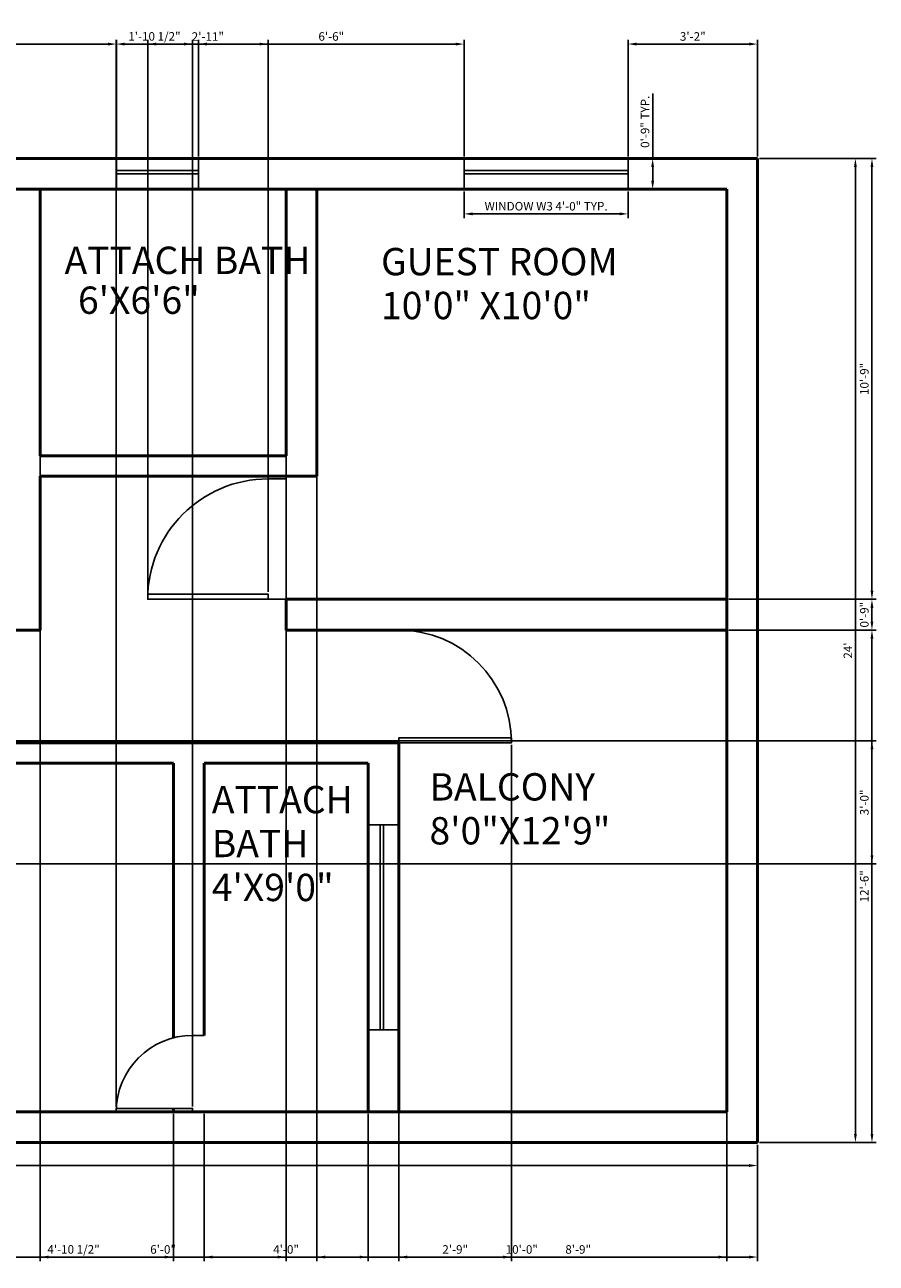
# Model space of a CAD drawing. Units: inches. Extents: x -5798 to 2718, y 1530 to 38999.
# Tile 2 of 4: x 2468 to 2718, y 1557 to 1919. Entities that reach past the tile are written whole.
import ezdxf

# ---------------------------------------------------------------- set-up
doc = ezdxf.new("R2010")
doc.units = ezdxf.units.IN
for name, color, linetype, lineweight in [('A-ANNO-DIMS', 2, 'Continuous', 18), ('A-AREA-IDEN', 3, 'Continuous', 18), ('A-DOOR', 3, 'Continuous', 25), ('A-GLAZ', 4, 'Continuous', 25), ('A-WALL', 7, 'Continuous', 50)]:
    doc.layers.add(name, color=color, linetype=linetype, lineweight=lineweight)
doc.styles.get("Standard").update_dxf_attribs({"font": 'arial.ttf'})
doc.dimstyles.new('Copy of ISO-25', dxfattribs={"dimtxt": 2.5, "dimasz": 2.5, "dimexe": 1.25, "dimexo": 0.625, "dimtad": 1, "dimdec": 1, "dimlunit": 4, "dimtxsty": 'Standard', "dimcen": 2.5, "dimadec": 0, "dimazin": 0, "dimtfac": 1, "dimtdec": 1, "dimtmove": 0, "dimatfit": 3, "dimfxl": 1, "dimarcsym": 0})

# ---------------------------------------------------------------- blocks, each defined once
blk = doc.blocks.new('*U2')
for p, q in [((0, 0), (0, -6)), ((40, 0), (40, -6))]:
    blk.add_line(p, q)
blk.add_lwpolyline([(0, 0), (0, 40), (1.75, 40), (1.75, 0)], close=True)
blk.add_arc((0, 0), 40, 0, 90)
blk = doc.blocks.new('*U7')
for p, q in [((0, 0), (0, 6)), ((40, 0), (40, 6))]:
    blk.add_line(p, q)
blk.add_lwpolyline([(0, 0), (0, -40), (1.75, -40), (1.75, 0)], close=True)
blk.add_arc((0, 0), 40, 270, 0)
blk = doc.blocks.new('*D15')
at = {"layer": 'A-ANNO-DIMS', "color": 0, "lineweight": -2, "transparency": 16777216}
for p, q in [((2683.52, 1880.03), (2712.8, 1880.03)), ((2711.55, 1877.53), (2711.55, 1594.53)), ((2683.52, 1592.03), (2712.8, 1592.03))]:
    blk.add_line(p, q, dxfattribs=at)
at = {"layer": 'A-ANNO-DIMS', "color": 0, "transparency": 16777216}
for points in [[(2711.14, 1877.53), (2711.97, 1877.53), (2711.55, 1880.03)], [(2711.14, 1594.53), (2711.97, 1594.53), (2711.55, 1592.03)]]:
    blk.add_solid(points, dxfattribs=at)
at = {"layer": 'Defpoints', "color": 0, "transparency": 16777216}
for p in [(2682.89, 1880.03), (2682.89, 1592.03), (2711.55, 1592.03)]:
    blk.add_point(p, dxfattribs=at)
at = {"layer": 'A-ANNO-DIMS', "color": 0, "transparency": 16777216, "insert": (2709.67, 1736.03), "char_height": 2.5, "attachment_point": 5, "rotation": 90}
blk.add_mtext("24'", dxfattribs=at)
blk = doc.blocks.new('*D16')
at = {"layer": 'A-ANNO-DIMS', "color": 0, "lineweight": -2, "transparency": 16777216}
for p, q in [((2042.98, 1591.41), (2042.98, 1584.06)), ((2682.89, 1591.41), (2682.89, 1584.06)), ((2045.48, 1585.31), (2680.39, 1585.31))]:
    blk.add_line(p, q, dxfattribs=at)
at = {"layer": 'A-ANNO-DIMS', "color": 0, "transparency": 16777216}
for points in [[(2045.48, 1585.73), (2045.48, 1584.89), (2042.98, 1585.31)], [(2680.39, 1585.73), (2680.39, 1584.89), (2682.89, 1585.31)]]:
    blk.add_solid(points, dxfattribs=at)
at = {"layer": 'Defpoints', "color": 0, "transparency": 16777216}
for p in [(2042.98, 1592.03), (2682.89, 1592.03), (2682.89, 1585.31)]:
    blk.add_point(p, dxfattribs=at)
at = {"layer": 'A-ANNO-DIMS', "color": 0, "transparency": 16777216, "insert": (2362.93, 1587.21), "char_height": 2.5, "attachment_point": 5}
blk.add_mtext('53\'-4"', dxfattribs=at)
blk = doc.blocks.new('WIN-48')
for p, q in [((0, 0), (0, 9)), ((0, 9), (48, 9)), ((48, 9), (48, 0)), ((0, 5.5), (48, 5.5)), ((0, 4.5), (48, 4.5))]:
    blk.add_line(p, q)
blk = doc.blocks.new('WIN-60')
for p, q in [((0, 0), (0, 9)), ((0, 9), (60, 9)), ((60, 9), (60, 0)), ((0, 4.5), (60, 4.5)), ((0, 3.5), (60, 3.5))]:
    blk.add_line(p, q)
blk = doc.blocks.new('WIN-24-B')
for p, q in [((0, 0), (0, 9)), ((0, 9), (24, 9)), ((24, 9), (24, 0)), ((0, 5.5), (24, 5.5)), ((0, 4.5), (24, 4.5))]:
    blk.add_line(p, q)
blk = doc.blocks.new('*D26')
at = {"layer": 'A-ANNO-DIMS', "color": 0, "lineweight": -2, "transparency": 16777216}
for p, q in [((2597, 1870.41), (2597, 1862.58)), ((2645, 1870.41), (2645, 1862.58)), ((2599.5, 1863.83), (2642.5, 1863.83))]:
    blk.add_line(p, q, dxfattribs=at)
at = {"layer": 'A-ANNO-DIMS', "color": 0, "transparency": 16777216}
for points in [[(2599.5, 1864.25), (2599.5, 1863.41), (2597, 1863.83)], [(2642.5, 1864.25), (2642.5, 1863.41), (2645, 1863.83)]]:
    blk.add_solid(points, dxfattribs=at)
at = {"layer": 'Defpoints', "color": 0, "transparency": 16777216}
for p in [(2597, 1871.03), (2645, 1871.03), (2645, 1863.83)]:
    blk.add_point(p, dxfattribs=at)
at = {"layer": 'A-ANNO-DIMS', "color": 0, "transparency": 16777216, "insert": (2621, 1865.75), "char_height": 2.5, "attachment_point": 5}
blk.add_mtext('WINDOW W3 4\'-0" TYP.', dxfattribs=at)
blk = doc.blocks.new('*D27')
at = {"layer": 'A-ANNO-DIMS', "color": 0, "lineweight": -2, "transparency": 16777216}
for p, q in [((2652.2, 1880.03), (2652.2, 1899.02)), ((2645.62, 1880.03), (2653.45, 1880.03)), ((2652.2, 1873.53), (2652.2, 1877.53)), ((2645.62, 1871.03), (2653.45, 1871.03))]:
    blk.add_line(p, q, dxfattribs=at)
at = {"layer": 'A-ANNO-DIMS', "color": 0, "transparency": 16777216}
for points in [[(2651.78, 1877.53), (2652.61, 1877.53), (2652.2, 1880.03)], [(2651.78, 1873.53), (2652.61, 1873.53), (2652.2, 1871.03)]]:
    blk.add_solid(points, dxfattribs=at)
at = {"layer": 'Defpoints', "color": 0, "transparency": 16777216}
for p in [(2645, 1880.03), (2652.2, 1880.03), (2645, 1871.03)]:
    blk.add_point(p, dxfattribs=at)
at = {"layer": 'A-ANNO-DIMS', "color": 0, "transparency": 16777216, "insert": (2650.29, 1890.78), "char_height": 2.5, "attachment_point": 5, "rotation": 90}
blk.add_mtext('0\'-9" TYP.', dxfattribs=at)
blk = doc.blocks.new('*D71')
at = {"layer": 'A-ANNO-DIMS', "color": 0, "lineweight": -2, "transparency": 16777216}
for p, q in [((2411.27, 1880.66), (2411.27, 1914.78)), ((2495.24, 1880.66), (2495.24, 1914.78)), ((2413.77, 1913.53), (2492.74, 1913.53))]:
    blk.add_line(p, q, dxfattribs=at)
at = {"layer": 'A-ANNO-DIMS', "color": 0, "transparency": 16777216}
for points in [[(2413.77, 1913.95), (2413.77, 1913.11), (2411.27, 1913.53)], [(2492.74, 1913.95), (2492.74, 1913.11), (2495.24, 1913.53)]]:
    blk.add_solid(points, dxfattribs=at)
at = {"layer": 'Defpoints', "color": 0, "transparency": 16777216}
for p in [(2495.24, 1913.53), (2411.27, 1880.03), (2495.24, 1880.03)]:
    blk.add_point(p, dxfattribs=at)
at = {"layer": 'A-ANNO-DIMS', "color": 0, "transparency": 16777216, "insert": (2453.26, 1915.43), "char_height": 2.5, "attachment_point": 5}
blk.add_mtext('7\'-0"', dxfattribs=at)
blk = doc.blocks.new('*D72')
at = {"layer": 'A-ANNO-DIMS', "color": 0, "lineweight": -2, "transparency": 16777216}
for p, q in [((2519.24, 1880.66), (2519.24, 1914.78)), ((2597, 1880.66), (2597, 1914.78)), ((2521.74, 1913.53), (2594.5, 1913.53))]:
    blk.add_line(p, q, dxfattribs=at)
at = {"layer": 'A-ANNO-DIMS', "color": 0, "transparency": 16777216}
for points in [[(2521.74, 1913.95), (2521.74, 1913.11), (2519.24, 1913.53)], [(2594.5, 1913.95), (2594.5, 1913.11), (2597, 1913.53)]]:
    blk.add_solid(points, dxfattribs=at)
at = {"layer": 'Defpoints', "color": 0, "transparency": 16777216}
for p in [(2597, 1913.53), (2519.24, 1880.03), (2597, 1880.03)]:
    blk.add_point(p, dxfattribs=at)
at = {"layer": 'A-ANNO-DIMS', "color": 0, "transparency": 16777216, "insert": (2558.12, 1915.43), "char_height": 2.5, "attachment_point": 5}
blk.add_mtext('6\'-6"', dxfattribs=at)
blk = doc.blocks.new('*D73')
at = {"layer": 'A-ANNO-DIMS', "color": 0, "lineweight": -2, "transparency": 16777216}
for p, q in [((2645, 1880.66), (2645, 1914.78)), ((2682.89, 1880.66), (2682.89, 1914.78)), ((2647.5, 1913.53), (2680.39, 1913.53))]:
    blk.add_line(p, q, dxfattribs=at)
at = {"layer": 'A-ANNO-DIMS', "color": 0, "transparency": 16777216}
for points in [[(2647.5, 1913.95), (2647.5, 1913.11), (2645, 1913.53)], [(2680.39, 1913.95), (2680.39, 1913.11), (2682.89, 1913.53)]]:
    blk.add_solid(points, dxfattribs=at)
at = {"layer": 'Defpoints', "color": 0, "transparency": 16777216}
for p in [(2682.89, 1913.53), (2645, 1880.03), (2682.89, 1880.03)]:
    blk.add_point(p, dxfattribs=at)
at = {"layer": 'A-ANNO-DIMS', "color": 0, "transparency": 16777216, "insert": (2663.94, 1915.43), "char_height": 2.5, "attachment_point": 5}
blk.add_mtext('3\'-2"', dxfattribs=at)
blk = doc.blocks.new('*D78')
at = {"layer": 'A-ANNO-DIMS', "color": 0, "lineweight": -2, "transparency": 16777216}
for p, q in [((2472.89, 1870.41), (2472.89, 1557.28)), ((2544.89, 1870.41), (2544.89, 1557.28)), ((2475.39, 1558.53), (2542.39, 1558.53))]:
    blk.add_line(p, q, dxfattribs=at)
at = {"layer": 'A-ANNO-DIMS', "color": 0, "transparency": 16777216}
for points in [[(2475.39, 1558.95), (2475.39, 1558.11), (2472.89, 1558.53)], [(2542.39, 1558.95), (2542.39, 1558.11), (2544.89, 1558.53)]]:
    blk.add_solid(points, dxfattribs=at)
at = {"layer": 'Defpoints', "color": 0, "transparency": 16777216}
for p in [(2472.89, 1871.03), (2544.89, 1871.03), (2544.89, 1558.53)]:
    blk.add_point(p, dxfattribs=at)
at = {"layer": 'A-ANNO-DIMS', "color": 0, "transparency": 16777216, "insert": (2508.89, 1560.43), "char_height": 2.5, "attachment_point": 5}
blk.add_mtext('6\'-0"', dxfattribs=at)
blk = doc.blocks.new('*D79')
at = {"layer": 'A-ANNO-DIMS', "color": 0, "lineweight": -2, "transparency": 16777216}
for p, q in [((2553.89, 1870.41), (2553.89, 1557.28)), ((2673.89, 1870.41), (2673.89, 1557.28)), ((2556.39, 1558.53), (2671.39, 1558.53))]:
    blk.add_line(p, q, dxfattribs=at)
at = {"layer": 'A-ANNO-DIMS', "color": 0, "transparency": 16777216}
for points in [[(2556.39, 1558.95), (2556.39, 1558.11), (2553.89, 1558.53)], [(2671.39, 1558.95), (2671.39, 1558.11), (2673.89, 1558.53)]]:
    blk.add_solid(points, dxfattribs=at)
at = {"layer": 'Defpoints', "color": 0, "transparency": 16777216}
for p in [(2553.89, 1871.03), (2673.89, 1871.03), (2673.89, 1558.53)]:
    blk.add_point(p, dxfattribs=at)
at = {"layer": 'A-ANNO-DIMS', "color": 0, "transparency": 16777216, "insert": (2613.89, 1560.43), "char_height": 2.5, "attachment_point": 5}
blk.add_mtext('10\'-0"', dxfattribs=at)
blk = doc.blocks.new('*D84')
at = {"layer": 'A-ANNO-DIMS', "color": 0, "lineweight": -2, "transparency": 16777216}
for p, q in [((2683.52, 1880.03), (2717.64, 1880.03)), ((2716.39, 1877.53), (2716.39, 1753.53)), ((2674.52, 1751.03), (2717.64, 1751.03))]:
    blk.add_line(p, q, dxfattribs=at)
at = {"layer": 'A-ANNO-DIMS', "color": 0, "transparency": 16777216}
for points in [[(2715.98, 1877.53), (2716.81, 1877.53), (2716.39, 1880.03)], [(2715.98, 1753.53), (2716.81, 1753.53), (2716.39, 1751.03)]]:
    blk.add_solid(points, dxfattribs=at)
at = {"layer": 'Defpoints', "color": 0, "transparency": 16777216}
for p in [(2682.89, 1880.03), (2673.89, 1751.03), (2716.39, 1751.03)]:
    blk.add_point(p, dxfattribs=at)
at = {"layer": 'A-ANNO-DIMS', "color": 0, "transparency": 16777216, "insert": (2714.49, 1815.53), "char_height": 2.5, "attachment_point": 5, "rotation": 90}
blk.add_mtext('10\'-9"', dxfattribs=at)
blk = doc.blocks.new('*D85')
at = {"layer": 'A-ANNO-DIMS', "color": 0, "lineweight": -2, "transparency": 16777216}
for p, q in [((2674.52, 1751.03), (2717.64, 1751.03)), ((2716.39, 1748.53), (2716.39, 1744.53)), ((2674.52, 1742.03), (2717.64, 1742.03))]:
    blk.add_line(p, q, dxfattribs=at)
at = {"layer": 'A-ANNO-DIMS', "color": 0, "transparency": 16777216}
for points in [[(2715.98, 1748.53), (2716.81, 1748.53), (2716.39, 1751.03)], [(2715.98, 1744.53), (2716.81, 1744.53), (2716.39, 1742.03)]]:
    blk.add_solid(points, dxfattribs=at)
at = {"layer": 'Defpoints', "color": 0, "transparency": 16777216}
for p in [(2673.89, 1751.03), (2673.89, 1742.03), (2716.39, 1742.03)]:
    blk.add_point(p, dxfattribs=at)
at = {"layer": 'A-ANNO-DIMS', "color": 0, "transparency": 16777216, "insert": (2714.49, 1746.53), "char_height": 2.5, "attachment_point": 5, "rotation": 90}
blk.add_mtext('0\'-9"', dxfattribs=at)
blk = doc.blocks.new('*D86')
at = {"layer": 'A-ANNO-DIMS', "color": 0, "lineweight": -2, "transparency": 16777216}
for p, q in [((2674.52, 1742.03), (2717.64, 1742.03)), ((2716.39, 1739.53), (2716.39, 1594.53)), ((2683.52, 1592.03), (2717.64, 1592.03))]:
    blk.add_line(p, q, dxfattribs=at)
at = {"layer": 'A-ANNO-DIMS', "color": 0, "transparency": 16777216}
for points in [[(2715.98, 1739.53), (2716.81, 1739.53), (2716.39, 1742.03)], [(2715.98, 1594.53), (2716.81, 1594.53), (2716.39, 1592.03)]]:
    blk.add_solid(points, dxfattribs=at)
at = {"layer": 'Defpoints', "color": 0, "transparency": 16777216}
for p in [(2673.89, 1742.03), (2682.89, 1592.03), (2716.39, 1592.03)]:
    blk.add_point(p, dxfattribs=at)
at = {"layer": 'A-ANNO-DIMS', "color": 0, "transparency": 16777216, "insert": (2714.49, 1667.03), "char_height": 2.5, "attachment_point": 5, "rotation": 90}
blk.add_mtext('12\'-6"', dxfattribs=at)
blk = doc.blocks.new('*D90')
at = {"layer": 'A-ANNO-DIMS', "color": 0, "lineweight": -2, "transparency": 16777216}
for p, q in [((2511.89, 1600.41), (2511.89, 1557.28)), ((2453.45, 1591.41), (2453.45, 1557.28)), ((2455.95, 1558.53), (2509.39, 1558.53))]:
    blk.add_line(p, q, dxfattribs=at)
at = {"layer": 'A-ANNO-DIMS', "color": 0, "transparency": 16777216}
for points in [[(2455.95, 1558.95), (2455.95, 1558.11), (2453.45, 1558.53)], [(2509.39, 1558.95), (2509.39, 1558.11), (2511.89, 1558.53)]]:
    blk.add_solid(points, dxfattribs=at)
at = {"layer": 'Defpoints', "color": 0, "transparency": 16777216}
for p in [(2511.89, 1601.03), (2453.45, 1592.03), (2511.89, 1558.53)]:
    blk.add_point(p, dxfattribs=at)
at = {"layer": 'A-ANNO-DIMS', "color": 0, "transparency": 16777216, "insert": (2482.67, 1560.45), "char_height": 2.5, "attachment_point": 5}
blk.add_mtext('4\'-10 1/2"', dxfattribs=at)
blk = doc.blocks.new('*D91')
at = {"layer": 'A-ANNO-DIMS', "color": 0, "lineweight": -2, "transparency": 16777216}
for p, q in [((2520.89, 1600.41), (2520.89, 1557.28)), ((2568.89, 1600.41), (2568.89, 1557.28)), ((2523.39, 1558.53), (2566.39, 1558.53))]:
    blk.add_line(p, q, dxfattribs=at)
at = {"layer": 'A-ANNO-DIMS', "color": 0, "transparency": 16777216}
for points in [[(2523.39, 1558.95), (2523.39, 1558.11), (2520.89, 1558.53)], [(2566.39, 1558.95), (2566.39, 1558.11), (2568.89, 1558.53)]]:
    blk.add_solid(points, dxfattribs=at)
at = {"layer": 'Defpoints', "color": 0, "transparency": 16777216}
for p in [(2520.89, 1601.03), (2568.89, 1601.03), (2568.89, 1558.53)]:
    blk.add_point(p, dxfattribs=at)
at = {"layer": 'A-ANNO-DIMS', "color": 0, "transparency": 16777216, "insert": (2544.89, 1560.43), "char_height": 2.5, "attachment_point": 5}
blk.add_mtext('4\'-0"', dxfattribs=at)
blk = doc.blocks.new('*D92')
at = {"layer": 'A-ANNO-DIMS', "color": 0, "lineweight": -2, "transparency": 16777216}
for p, q in [((2577.89, 1600.41), (2577.89, 1557.28)), ((2682.89, 1591.41), (2682.89, 1557.28)), ((2580.39, 1558.53), (2680.39, 1558.53))]:
    blk.add_line(p, q, dxfattribs=at)
at = {"layer": 'A-ANNO-DIMS', "color": 0, "transparency": 16777216}
for points in [[(2580.39, 1558.95), (2580.39, 1558.11), (2577.89, 1558.53)], [(2680.39, 1558.95), (2680.39, 1558.11), (2682.89, 1558.53)]]:
    blk.add_solid(points, dxfattribs=at)
at = {"layer": 'Defpoints', "color": 0, "transparency": 16777216}
for p in [(2577.89, 1601.03), (2682.89, 1592.03), (2682.89, 1558.53)]:
    blk.add_point(p, dxfattribs=at)
at = {"layer": 'A-ANNO-DIMS', "color": 0, "transparency": 16777216, "insert": (2630.39, 1560.43), "char_height": 2.5, "attachment_point": 5}
blk.add_mtext('8\'-9"', dxfattribs=at)
blk = doc.blocks.new('*D94')
at = {"layer": 'A-ANNO-DIMS', "color": 0, "lineweight": -2, "transparency": 16777216}
for p, q in [((2102.18, 1709.6), (2717.64, 1709.6)), ((2716.39, 1707.1), (2716.39, 1676.07)), ((2102.18, 1673.57), (2717.64, 1673.57))]:
    blk.add_line(p, q, dxfattribs=at)
at = {"layer": 'A-ANNO-DIMS', "color": 0, "transparency": 16777216}
for points in [[(2715.98, 1707.1), (2716.81, 1707.1), (2716.39, 1709.6)], [(2715.98, 1676.07), (2716.81, 1676.07), (2716.39, 1673.57)]]:
    blk.add_solid(points, dxfattribs=at)
at = {"layer": 'Defpoints', "color": 0, "transparency": 16777216}
for p in [(2101.55, 1709.6), (2101.55, 1673.57), (2716.39, 1673.57)]:
    blk.add_point(p, dxfattribs=at)
at = {"layer": 'A-ANNO-DIMS', "color": 0, "transparency": 16777216, "insert": (2714.49, 1691.59), "char_height": 2.5, "attachment_point": 5, "rotation": 90}
blk.add_mtext('3\'-0"', dxfattribs=at)
blk = doc.blocks.new('*D98')
at = {"layer": 'A-ANNO-DIMS', "color": 0, "lineweight": -2, "transparency": 16777216}
for p, q in [((2504.38, 1753.2), (2504.38, 1914.78)), ((2539.61, 1753.2), (2539.61, 1914.78)), ((2506.88, 1913.53), (2537.11, 1913.53))]:
    blk.add_line(p, q, dxfattribs=at)
at = {"layer": 'A-ANNO-DIMS', "color": 0, "transparency": 16777216}
for points in [[(2506.88, 1913.95), (2506.88, 1913.11), (2504.38, 1913.53)], [(2537.11, 1913.95), (2537.11, 1913.11), (2539.61, 1913.53)]]:
    blk.add_solid(points, dxfattribs=at)
at = {"layer": 'Defpoints', "color": 0, "transparency": 16777216}
for p in [(2539.61, 1913.53), (2504.38, 1752.57), (2539.61, 1752.57)]:
    blk.add_point(p, dxfattribs=at)
at = {"layer": 'A-ANNO-DIMS', "color": 0, "transparency": 16777216, "insert": (2521.99, 1915.41), "char_height": 2.5, "attachment_point": 5}
blk.add_mtext('2\'-11"', dxfattribs=at)
blk = doc.blocks.new('*D99')
at = {"layer": 'A-ANNO-DIMS', "color": 0, "lineweight": -2, "transparency": 16777216}
for p, q in [((2577.89, 1708.41), (2577.89, 1557.28)), ((2610.9, 1708.41), (2610.9, 1557.28)), ((2580.39, 1558.53), (2608.4, 1558.53))]:
    blk.add_line(p, q, dxfattribs=at)
at = {"layer": 'A-ANNO-DIMS', "color": 0, "transparency": 16777216}
for points in [[(2580.39, 1558.95), (2580.39, 1558.11), (2577.89, 1558.53)], [(2608.4, 1558.95), (2608.4, 1558.11), (2610.9, 1558.53)]]:
    blk.add_solid(points, dxfattribs=at)
at = {"layer": 'Defpoints', "color": 0, "transparency": 16777216}
for p in [(2577.89, 1709.03), (2610.9, 1709.03), (2610.9, 1558.53)]:
    blk.add_point(p, dxfattribs=at)
at = {"layer": 'A-ANNO-DIMS', "color": 0, "transparency": 16777216, "insert": (2594.39, 1560.43), "char_height": 2.5, "attachment_point": 5}
blk.add_mtext('2\'-9"', dxfattribs=at)
blk = doc.blocks.new('*D100')
at = {"layer": 'A-ANNO-DIMS', "color": 0, "lineweight": -2, "transparency": 16777216}
for p, q in [((2495.16, 1602.63), (2495.16, 1914.78)), ((2517.54, 1602.63), (2517.54, 1914.78)), ((2497.66, 1913.53), (2515.04, 1913.53))]:
    blk.add_line(p, q, dxfattribs=at)
at = {"layer": 'A-ANNO-DIMS', "color": 0, "transparency": 16777216}
for points in [[(2497.66, 1913.95), (2497.66, 1913.11), (2495.16, 1913.53)], [(2515.04, 1913.95), (2515.04, 1913.11), (2517.54, 1913.53)]]:
    blk.add_solid(points, dxfattribs=at)
at = {"layer": 'Defpoints', "color": 0, "transparency": 16777216}
for p in [(2517.54, 1913.53), (2495.16, 1602.01), (2517.54, 1602.01)]:
    blk.add_point(p, dxfattribs=at)
at = {"layer": 'A-ANNO-DIMS', "color": 0, "transparency": 16777216, "insert": (2506.35, 1915.45), "char_height": 2.5, "attachment_point": 5}
blk.add_mtext('1\'-10 1/2"', dxfattribs=at)

msp = doc.modelspace()

# ---------------------------------------------------------------- linework, layer by layer
at = {"layer": 'A-WALL'}
for p, q in [((2042.98, 1880.03), (2682.89, 1880.03)), ((2682.89, 1880.03), (2682.89, 1592.03)), ((2051.98, 1871.03), (2673.89, 1871.03)), ((2544.89, 1871.03), (2472.89, 1871.03)), ((2472.89, 1871.03), (2472.89, 1793.03)), ((2472.89, 1871.03), (2495.24, 1871.03)), ((2544.89, 1793.03), (2544.89, 1871.03)), ((2544.89, 1871.03), (2544.89, 1793.03)), ((2673.89, 1871.03), (2553.89, 1871.03)), ((2553.89, 1871.03), (2553.89, 1787.03)), ((2673.89, 1871.03), (2673.89, 1601.03)), ((2544.89, 1793.03), (2472.89, 1793.03)), ((2472.89, 1787.03), (2544.89, 1787.03)), ((2472.89, 1787.03), (2472.89, 1742.03)), ((2544.89, 1787.03), (2553.89, 1787.03)), ((2553.89, 1751.03), (2544.89, 1751.03)), ((2673.89, 1751.03), (2544.89, 1751.03)), ((2544.89, 1751.03), (2544.89, 1742.03)), ((2673.89, 1742.03), (2673.89, 1751.03)), ((2472.89, 1742.03), (2463.89, 1742.03)), ((2544.89, 1742.03), (2673.89, 1742.03)), ((2395.48, 1709.03), (2577.89, 1709.03)), ((2577.89, 1601.03), (2577.89, 1709.03)), ((2577.89, 1709.03), (2577.89, 1703.03)), ((2511.89, 1703.03), (2395.48, 1703.03)), ((2511.89, 1703.03), (2511.89, 1622.68)), ((2520.89, 1623.4), (2520.89, 1703.03)), ((2568.89, 1703.03), (2520.89, 1703.03)), ((2568.89, 1703.03), (2568.89, 1601.03)), ((2568.89, 1703.03), (2568.89, 1685.07)), ((2309.98, 1601.03), (2673.89, 1601.03)), ((2511.89, 1602.01), (2511.89, 1601.03)), ((2568.89, 1601.03), (2520.89, 1601.03)), ((2673.89, 1601.03), (2577.89, 1601.03)), ((2237.98, 1592.03), (2673.89, 1592.03)), ((2673.89, 1592.03), (2682.89, 1592.03))]:
    msp.add_line(p, q, dxfattribs=at)

# ---------------------------------------------------------------- block references
at = {"layer": 'A-DOOR', "rotation": 90}
for name, p, xscale, yscale, zscale in [('*U2', (2539.61, 1751.03), 0.8808171385769682, 0.8808171385769682, 0.8808171385769682), ('*U7', (2577.89, 1709.03), 0.8250422112901006, 0.8250422112901006, 0.8250422112901006), ('*U2', (2517.54, 1601.03), 0.559347909087562, 0.559347909087562, 0.559347909087562)]:
    msp.add_blockref(name, p, dxfattribs=dict(at, xscale=xscale, yscale=yscale, zscale=zscale))
at = {"layer": 'A-GLAZ'}
for name, p in [('WIN-24-B', (2495.24, 1871.03)), ('WIN-48', (2597, 1871.03))]:
    msp.add_blockref(name, p, dxfattribs=at)
at = {"layer": 'A-GLAZ', "rotation": 269.9999999999998}
msp.add_blockref('WIN-60', (2568.89, 1685.07), dxfattribs=at)

# ---------------------------------------------------------------- texts
at = {"layer": 'A-AREA-IDEN'}
for s, p in [('ATTACH BATH', (2480.04, 1846.24)), ('GUEST ROOM', (2572.68, 1845.86)), ('6\'X6\'6"', (2483.98, 1834.57)), ('10\'0" X10\'0"', (2572.68, 1833.01)), ('BALCONY', (2586.87, 1692.14)), ('ATTACH', (2523.15, 1688.41)), ('8\'0"X12\'9"', (2586.87, 1679.29)), ('BATH', (2523.15, 1675.56)), ('4\'X9\'0"', (2523.15, 1662.7))]:
    msp.add_text(s, height=8, dxfattribs=at).set_placement(p)

# ---------------------------------------------------------------- dimensions: what is measured, and where the dimension line sits
at = {"layer": 'A-ANNO-DIMS'}
for base, p1, p2, override, picture, middle in [((2517.54, 1913.53), (2495.16, 1602.01), (2517.54, 1602.01), {"dimdec": 1, "dimlfac": 1, "dimrnd": 0, "dimzin": 1, "dimdsep": 46, "dimlunit": 4, "dimfrac": 2}, '*D100', (2506.35, 1915.45)), ((2495.24, 1913.53), (2411.27, 1880.03), (2495.24, 1880.03), {"dimdec": 1, "dimlfac": 1, "dimrnd": 0, "dimzin": 1, "dimdsep": 46, "dimlunit": 4, "dimfrac": 2}, '*D71', (2453.26, 1915.43)), ((2539.61, 1913.53), (2504.38, 1752.57), (2539.61, 1752.57), {"dimdec": 1, "dimlfac": 1, "dimrnd": 0, "dimzin": 1, "dimdsep": 46, "dimlunit": 4, "dimfrac": 2}, '*D98', (2521.99, 1915.41)), ((2597, 1913.53), (2519.24, 1880.03), (2597, 1880.03), {"dimdec": 1, "dimlfac": 1, "dimrnd": 0, "dimzin": 1, "dimdsep": 46, "dimlunit": 4, "dimfrac": 2}, '*D72', (2558.12, 1915.43)), ((2682.89, 1913.53), (2645, 1880.03), (2682.89, 1880.03), {"dimdec": 1, "dimlfac": 1, "dimrnd": 0, "dimzin": 1, "dimdsep": 46, "dimlunit": 4, "dimfrac": 2}, '*D73', (2663.94, 1915.43)), ((2544.89, 1558.53), (2472.89, 1871.03), (2544.89, 1871.03), {"dimdec": 1, "dimlfac": 1, "dimrnd": 0, "dimzin": 1, "dimdsep": 46, "dimlunit": 4, "dimfrac": 2}, '*D78', (2508.89, 1560.43)), ((2673.89, 1558.53), (2553.89, 1871.03), (2673.89, 1871.03), {"dimdec": 1, "dimlfac": 1, "dimrnd": 0, "dimzin": 1, "dimdsep": 46, "dimlunit": 4, "dimfrac": 2}, '*D79', (2613.89, 1560.43)), ((2610.9, 1558.53), (2577.89, 1709.03), (2610.9, 1709.03), {"dimdec": 1, "dimlfac": 1, "dimrnd": 0, "dimzin": 1, "dimdsep": 46, "dimlunit": 4, "dimfrac": 2}, '*D99', (2594.39, 1560.43)), ((2511.89, 1558.53), (2453.45, 1592.03), (2511.89, 1601.03), {"dimdec": 1, "dimlfac": 1, "dimrnd": 0, "dimzin": 1, "dimdsep": 46, "dimlunit": 4, "dimfrac": 2}, '*D90', (2482.67, 1560.45)), ((2568.89, 1558.53), (2520.89, 1601.03), (2568.89, 1601.03), {"dimdec": 1, "dimlfac": 1, "dimrnd": 0, "dimzin": 1, "dimdsep": 46, "dimlunit": 4, "dimfrac": 2}, '*D91', (2544.89, 1560.43)), ((2682.89, 1558.53), (2577.89, 1601.03), (2682.89, 1592.03), {"dimdec": 1, "dimlfac": 1, "dimrnd": 0, "dimzin": 1, "dimdsep": 46, "dimlunit": 4, "dimfrac": 2}, '*D92', (2630.39, 1560.43)), ((2682.89, 1585.31), (2042.98, 1592.03), (2682.89, 1592.03), {"dimclrd": 0, "dimclre": 0, "dimclrt": 0}, '*D16', (2362.93, 1587.21))]:
    dim = msp.add_linear_dim(base=base, p1=p1, p2=p2, dimstyle='Copy of ISO-25', override=override, dxfattribs=at)
    dim.commit()
    dim.dimension.update_dxf_attribs({"geometry": picture, "text_midpoint": middle})
dim = msp.add_linear_dim(base=(2652.2, 1880.03), p1=(2645, 1871.03), p2=(2645, 1880.03), angle=90, text='<> TYP.', dimstyle='Copy of ISO-25', override={"dimdec": 1, "dimrnd": 0, "dimzin": 1, "dimlunit": 4, "dimfrac": 2}, dxfattribs=at)
dim.commit()
dim.dimension.update_dxf_attribs({"geometry": '*D27', "text_midpoint": (2650.29, 1890.78)})
for base, p1, p2, picture, middle in [((2716.39, 1751.03), (2682.89, 1880.03), (2673.89, 1751.03), '*D84', (2714.49, 1815.53)), ((2716.39, 1742.03), (2673.89, 1751.03), (2673.89, 1742.03), '*D85', (2714.49, 1746.53)), ((2716.39, 1592.03), (2673.89, 1742.03), (2682.89, 1592.03), '*D86', (2714.49, 1667.03)), ((2716.39, 1673.57), (2101.55, 1709.6), (2101.55, 1673.57), '*D94', (2714.49, 1691.59))]:
    dim = msp.add_linear_dim(base=base, p1=p1, p2=p2, angle=90, dimstyle='Copy of ISO-25', override={"dimdec": 1, "dimlfac": 1, "dimrnd": 0, "dimzin": 1, "dimdsep": 46, "dimlunit": 4, "dimfrac": 2}, dxfattribs=at)
    dim.commit()
    dim.dimension.update_dxf_attribs({"geometry": picture, "text_midpoint": middle})
dim = msp.add_aligned_dim(p1=(2682.89, 1880.03), p2=(2682.89, 1592.03), distance=28.66, dimstyle='Copy of ISO-25', override={"dimclrd": 0, "dimclre": 0, "dimclrt": 0}, dxfattribs=at)
dim.commit()
dim.dimension.update_dxf_attribs({"geometry": '*D15', "text_midpoint": (2709.67, 1736.03)})
dim = msp.add_linear_dim(base=(2645, 1863.83), p1=(2597, 1871.03), p2=(2645, 1871.03), text='WINDOW W3 <> TYP.', dimstyle='Copy of ISO-25', override={"dimdec": 1, "dimrnd": 0, "dimzin": 1, "dimlunit": 4, "dimfrac": 2}, dxfattribs=at)
dim.commit()
dim.dimension.update_dxf_attribs({"geometry": '*D26', "text_midpoint": (2621, 1865.75)})

doc.saveas('drawing.dxf')
